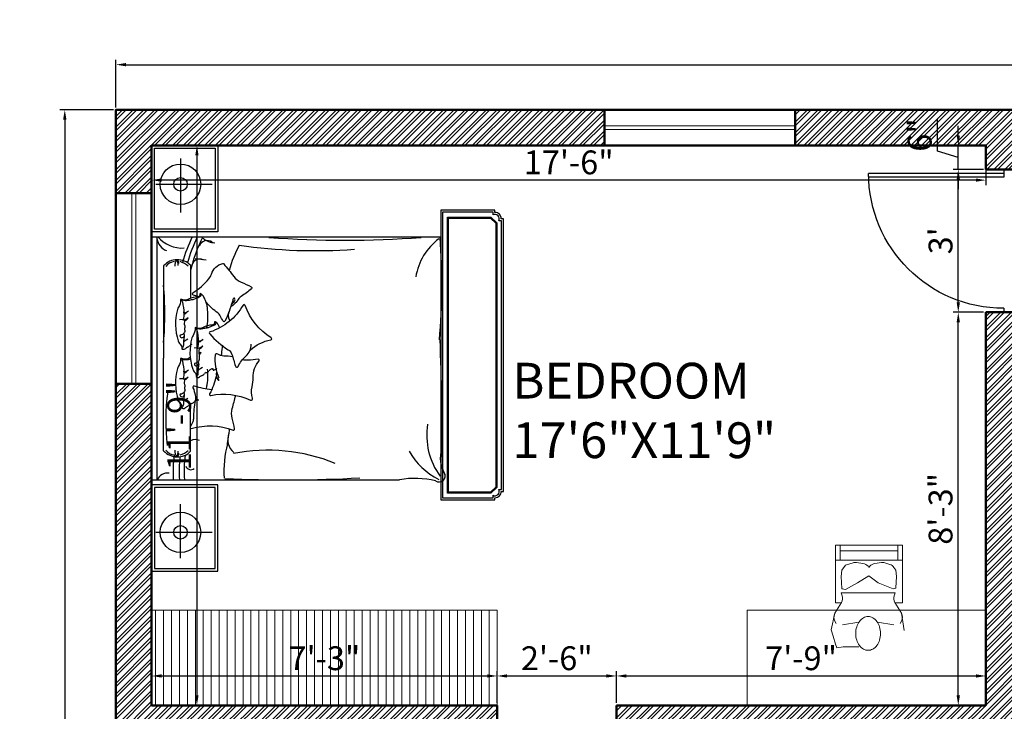
# Model space of a CAD drawing. Units: inches. Extents: x 3590 to 5167, y 65 to 1917.
# Tile 10 of 100: x 4396 to 4644, y 438 to 612. Entities that reach past the tile are written whole.
import ezdxf

# ---------------------------------------------------------------- set-up
doc = ezdxf.new("R2010")
doc.units = ezdxf.units.IN
for name, color, linetype, lineweight in [('A-ANNO-DIMS', 2, 'Continuous', 18), ('A-AREA-IDEN', 7, 'Continuous', 18), ('A-DOOR', 3, 'Continuous', 25), ('A-FURN', 21, 'Continuous', 18), ('A-GLAZ', 4, 'Continuous', 18), ('A-WALL', 7, 'Continuous', 50), ('A-WALL-PATT', 251, 'Continuous', 13)]:
    doc.layers.add(name, color=color, linetype=linetype, lineweight=lineweight)
for name, color, linetype in [('FUR', 42, 'Continuous'), ('HA-FUR', 8, 'Continuous'), ('HA-P', 8, 'Continuous'), ('SAN', 5, 'Continuous'), ('wood', 26, 'Continuous')]:
    doc.layers.add(name, color=color, linetype=linetype)
doc.styles.get("Standard").update_dxf_attribs({"font": 'arial.ttf'})
doc.dimstyles.new('ISO-25', dxfattribs={"dimtxt": 9, "dimasz": 2.5, "dimexe": 1.25, "dimexo": 0.625, "dimtad": 1, "dimdec": 1, "dimlunit": 3, "dimtxsty": 'Standard', "dimcen": 2.5, "dimadec": 0, "dimazin": 0, "dimtfac": 1, "dimtdec": 1, "dimtmove": 0, "dimatfit": 3, "dimfxl": 1, "dimarcsym": 0})

# ---------------------------------------------------------------- blocks, each defined once
blk = doc.blocks.new('*D279')
at = {"layer": 'A-ANNO-DIMS', "color": 0, "lineweight": -2, "transparency": 16777216}
for p, q in [((4420.27, 589.68), (4420.27, 601.68)), ((4422.77, 600.43), (5077.77, 600.43)), ((5080.27, 589.68), (5080.27, 601.68))]:
    blk.add_line(p, q, dxfattribs=at)
at = {"layer": 'A-ANNO-DIMS', "color": 0, "transparency": 16777216}
for points in [[(4422.77, 600.84), (4422.77, 600.01), (4420.27, 600.43)], [(5077.77, 600.84), (5077.77, 600.01), (5080.27, 600.43)]]:
    blk.add_solid(points, dxfattribs=at)
at = {"layer": 'Defpoints', "color": 0, "transparency": 16777216}
for p in [(5080.27, 600.43), (4420.27, 589.06), (5080.27, 589.06)]:
    blk.add_point(p, dxfattribs=at)
at = {"layer": 'A-ANNO-DIMS', "color": 0, "transparency": 16777216, "insert": (4750.27, 605.63), "char_height": 9, "attachment_point": 5}
blk.add_mtext("55'", dxfattribs=at)
blk = doc.blocks.new('*D280')
at = {"layer": 'A-ANNO-DIMS', "color": 0, "lineweight": -2, "transparency": 16777216}
for p, q in [((4419.65, 589.06), (4406.15, 589.06)), ((4407.4, 586.56), (4407.4, 111.56)), ((4419.65, 109.06), (4406.15, 109.06))]:
    blk.add_line(p, q, dxfattribs=at)
at = {"layer": 'A-ANNO-DIMS', "color": 0, "transparency": 16777216}
for points in [[(4406.98, 586.56), (4407.82, 586.56), (4407.4, 589.06)], [(4406.98, 111.56), (4407.82, 111.56), (4407.4, 109.06)]]:
    blk.add_solid(points, dxfattribs=at)
at = {"layer": 'Defpoints', "color": 0, "transparency": 16777216}
for p in [(4420.27, 589.06), (4407.4, 109.06), (4420.27, 109.06)]:
    blk.add_point(p, dxfattribs=at)
at = {"layer": 'A-ANNO-DIMS', "color": 0, "transparency": 16777216, "insert": (4402.18, 349.06), "char_height": 9, "attachment_point": 5, "rotation": 90}
blk.add_mtext("40'", dxfattribs=at)
blk = doc.blocks.new('D1')
for p, q in [((1, 0), (1, 34)), ((2, 0), (2, 33.99)), ((0, 0), (2, 0)), ((35, 0), (36, 0))]:
    blk.add_line(p, q)
at = {"ltscale": 0.5}
blk.add_arc((1, 0), 34, 0, 90, dxfattribs=at)
blk = doc.blocks.new('*D222')
at = {"layer": 'A-ANNO-DIMS', "color": 0, "lineweight": -2, "transparency": 16777216}
for p, q in [((4429.27, 579.43), (4429.27, 570.1)), ((4639.27, 579.43), (4639.27, 570.1)), ((4636.77, 571.35), (4431.77, 571.35))]:
    blk.add_line(p, q, dxfattribs=at)
at = {"layer": 'A-ANNO-DIMS', "color": 0, "transparency": 16777216}
for points in [[(4431.77, 571.77), (4431.77, 570.94), (4429.27, 571.35)], [(4636.77, 571.77), (4636.77, 570.94), (4639.27, 571.35)]]:
    blk.add_solid(points, dxfattribs=at)
at = {"layer": 'Defpoints', "color": 0, "transparency": 16777216}
for p in [(4429.27, 580.06), (4639.27, 580.06), (4429.27, 571.35)]:
    blk.add_point(p, dxfattribs=at)
at = {"layer": 'A-ANNO-DIMS', "color": 0, "transparency": 16777216, "insert": (4534.27, 575.04), "char_height": 6, "attachment_point": 5}
blk.add_mtext('17\'-6"', dxfattribs=at)
blk = doc.blocks.new('*D223')
at = {"layer": 'A-ANNO-DIMS', "color": 0, "lineweight": -2, "transparency": 16777216}
for p, q in [((4429.9, 580.06), (4441.91, 580.06)), ((4440.66, 577.56), (4440.66, 441.56)), ((4429.9, 439.06), (4441.91, 439.06))]:
    blk.add_line(p, q, dxfattribs=at)
at = {"layer": 'A-ANNO-DIMS', "color": 0, "transparency": 16777216}
for points in [[(4440.24, 577.56), (4441.08, 577.56), (4440.66, 580.06)], [(4440.24, 441.56), (4441.08, 441.56), (4440.66, 439.06)]]:
    blk.add_solid(points, dxfattribs=at)
at = {"layer": 'Defpoints', "color": 0, "transparency": 16777216}
for p in [(4429.27, 580.06), (4429.27, 439.06), (4440.66, 439.06)]:
    blk.add_point(p, dxfattribs=at)
at = {"layer": 'A-ANNO-DIMS', "color": 0, "transparency": 16777216, "insert": (4436.97, 509.56), "char_height": 6, "attachment_point": 5, "rotation": 90}
blk.add_mtext('11\'-9"', dxfattribs=at)
blk = doc.blocks.new('*D274')
at = {"layer": 'A-ANNO-DIMS', "color": 0, "lineweight": -2, "transparency": 16777216}
for p, q in [((4429.27, 439.68), (4429.27, 447.71)), ((4431.77, 446.46), (4513.77, 446.46)), ((4516.27, 439.68), (4516.27, 447.71))]:
    blk.add_line(p, q, dxfattribs=at)
at = {"layer": 'A-ANNO-DIMS', "color": 0, "transparency": 16777216}
for points in [[(4431.77, 446.88), (4431.77, 446.05), (4429.27, 446.46)], [(4513.77, 446.88), (4513.77, 446.05), (4516.27, 446.46)]]:
    blk.add_solid(points, dxfattribs=at)
at = {"layer": 'Defpoints', "color": 0, "transparency": 16777216}
for p in [(4516.27, 446.46), (4429.27, 439.06), (4516.27, 439.06)]:
    blk.add_point(p, dxfattribs=at)
at = {"layer": 'A-ANNO-DIMS', "color": 0, "transparency": 16777216, "insert": (4472.77, 450.15), "char_height": 6, "attachment_point": 5}
blk.add_mtext('7\'-3"', dxfattribs=at)
blk = doc.blocks.new('*D275')
at = {"layer": 'A-ANNO-DIMS', "color": 0, "lineweight": -2, "transparency": 16777216}
for p, q in [((4516.27, 439.68), (4516.27, 447.71)), ((4518.77, 446.46), (4543.77, 446.46)), ((4546.27, 439.68), (4546.27, 447.71))]:
    blk.add_line(p, q, dxfattribs=at)
at = {"layer": 'A-ANNO-DIMS', "color": 0, "transparency": 16777216}
for points in [[(4518.77, 446.88), (4518.77, 446.05), (4516.27, 446.46)], [(4543.77, 446.88), (4543.77, 446.05), (4546.27, 446.46)]]:
    blk.add_solid(points, dxfattribs=at)
at = {"layer": 'Defpoints', "color": 0, "transparency": 16777216}
for p in [(4546.27, 446.46), (4516.27, 439.06), (4546.27, 439.06)]:
    blk.add_point(p, dxfattribs=at)
at = {"layer": 'A-ANNO-DIMS', "color": 0, "transparency": 16777216, "insert": (4531.27, 450.15), "char_height": 6, "attachment_point": 5}
blk.add_mtext('2\'-6"', dxfattribs=at)
blk = doc.blocks.new('*D276')
at = {"layer": 'A-ANNO-DIMS', "color": 0, "lineweight": -2, "transparency": 16777216}
for p, q in [((4546.27, 439.68), (4546.27, 447.71)), ((4548.77, 446.46), (4636.77, 446.46)), ((4639.27, 439.68), (4639.27, 447.71))]:
    blk.add_line(p, q, dxfattribs=at)
at = {"layer": 'A-ANNO-DIMS', "color": 0, "transparency": 16777216}
for points in [[(4548.77, 446.88), (4548.77, 446.05), (4546.27, 446.46)], [(4636.77, 446.88), (4636.77, 446.05), (4639.27, 446.46)]]:
    blk.add_solid(points, dxfattribs=at)
at = {"layer": 'Defpoints', "color": 0, "transparency": 16777216}
for p in [(4639.27, 446.46), (4546.27, 439.06), (4639.27, 439.06)]:
    blk.add_point(p, dxfattribs=at)
at = {"layer": 'A-ANNO-DIMS', "color": 0, "transparency": 16777216, "insert": (4592.77, 450.15), "char_height": 6, "attachment_point": 5}
blk.add_mtext('7\'-9"', dxfattribs=at)
blk = doc.blocks.new('*D277')
at = {"layer": 'A-ANNO-DIMS', "color": 0, "lineweight": -2, "transparency": 16777216}
for p, q in [((4638.65, 538.06), (4631.09, 538.06)), ((4632.34, 441.56), (4632.34, 535.56)), ((4638.65, 439.06), (4631.09, 439.06))]:
    blk.add_line(p, q, dxfattribs=at)
at = {"layer": 'A-ANNO-DIMS', "color": 0, "transparency": 16777216}
for points in [[(4631.93, 535.56), (4632.76, 535.56), (4632.34, 538.06)], [(4631.93, 441.56), (4632.76, 441.56), (4632.34, 439.06)]]:
    blk.add_solid(points, dxfattribs=at)
at = {"layer": 'Defpoints', "color": 0, "transparency": 16777216}
for p in [(4632.34, 538.06), (4639.27, 538.06), (4639.27, 439.06)]:
    blk.add_point(p, dxfattribs=at)
at = {"layer": 'A-ANNO-DIMS', "color": 0, "transparency": 16777216, "insert": (4628.65, 488.56), "char_height": 6, "attachment_point": 5, "rotation": 90}
blk.add_mtext('8\'-3"', dxfattribs=at)
blk = doc.blocks.new('*D278')
at = {"layer": 'A-ANNO-DIMS', "color": 0, "lineweight": -2, "transparency": 16777216}
for p, q in [((4638.65, 574.06), (4631.09, 574.06)), ((4632.34, 540.56), (4632.34, 571.56)), ((4638.65, 538.06), (4631.09, 538.06))]:
    blk.add_line(p, q, dxfattribs=at)
at = {"layer": 'A-ANNO-DIMS', "color": 0, "transparency": 16777216}
for points in [[(4631.93, 571.56), (4632.76, 571.56), (4632.34, 574.06)], [(4631.93, 540.56), (4632.76, 540.56), (4632.34, 538.06)]]:
    blk.add_solid(points, dxfattribs=at)
at = {"layer": 'Defpoints', "color": 0, "transparency": 16777216}
for p in [(4632.34, 574.06), (4639.27, 574.06), (4639.27, 538.06)]:
    blk.add_point(p, dxfattribs=at)
at = {"layer": 'A-ANNO-DIMS', "color": 0, "transparency": 16777216, "insert": (4628.65, 556.06), "char_height": 6, "attachment_point": 5, "rotation": 90}
blk.add_mtext("3'", dxfattribs=at)
blk = doc.blocks.new('*D269')
at = {"layer": 'A-ANNO-DIMS', "color": 0, "lineweight": -2, "transparency": 16777216}
for p, q in [((4627.09, 578.64), (4627.09, 586.81)), ((4632.34, 582.56), (4632.34, 585.06)), ((4638.65, 580.06), (4631.09, 580.06)), ((4632.34, 574.06), (4632.34, 580.06)), ((4632.34, 574.06), (4632.34, 580.06)), ((4632.34, 577.06), (4627.09, 578.64)), ((4638.65, 574.06), (4631.09, 574.06)), ((4632.34, 571.56), (4632.34, 569.06))]:
    blk.add_line(p, q, dxfattribs=at)
at = {"layer": 'A-ANNO-DIMS', "color": 0, "transparency": 16777216}
for points in [[(4631.93, 582.56), (4632.76, 582.56), (4632.34, 580.06)], [(4631.93, 571.56), (4632.76, 571.56), (4632.34, 574.06)]]:
    blk.add_solid(points, dxfattribs=at)
at = {"layer": 'Defpoints', "color": 0, "transparency": 16777216}
for p in [(4632.34, 580.06), (4639.27, 580.06), (4639.27, 574.06)]:
    blk.add_point(p, dxfattribs=at)
at = {"layer": 'A-ANNO-DIMS', "color": 0, "transparency": 16777216, "insert": (4623.4, 582.72), "char_height": 6, "attachment_point": 5, "rotation": 90}
blk.add_mtext('6"', dxfattribs=at)
blk = doc.blocks.new('A$C0A42580C')
at = {"layer": 'SAN'}
for p, q in [((0.2873, 0.0301), (0.2873, 0.4484)), ((2.8678, 0.0301), (2.8678, 0.4484)), ((0.0949, 0.2135), (0.4958, 0.2135)), ((3.0601, 0.2135), (2.6592, 0.2135))]:
    blk.add_line(p, q, dxfattribs=at)
for centre, radius in [((0.2873, 0.2135), 0.15), ((2.8678, 0.2135), 0.15), ((0.2873, 0.2135), 0.05), ((2.8678, 0.2135), 0.05)]:
    blk.add_circle(centre, radius, dxfattribs=at)
at = {"layer": 'wood'}
for p, q in [((0.6775, 0.8851), (0.6775, 2.1392)), ((2.4775, 0.8016), (2.4775, 1.838)), ((2.4775, 0), (2.4775, 0.8016)), ((1.6633, 0.3438), (1.6434, 0.3761)), ((1.5, 0.3423), (1.5016, 0.3142)), ((0.888, 0.289), (1.1327, 0.289)), ((1.2906, 0.2348), (1.2921, 0.2067)), ((1.4538, 0.2362), (1.434, 0.2685)), ((1.7287, 0.2348), (1.7302, 0.2067)), ((1.8919, 0.2362), (1.8721, 0.2685)), ((2.267, 0.289), (1.9163, 0.289)), ((0.8909, 0.089), (1.5775, 0.089)), ((2.2642, 0.089), (1.5775, 0.089)), ((0.6775, 0.039), (2.4775, 0.039)), ((0.6775, 0), (2.4775, 0))]:
    blk.add_line(p, q, dxfattribs=at)
blk.add_lwpolyline([(0.6775, 0), (0.6775, 0.8851)], dxfattribs=at)
for points in [[(1.516, 0.7294, -0.128392), (1.4401, 0.8834, 0.70791), (1.427, 0.8863, -0.16964), (1.1848, 0.6919, 0.664036), (1.184, 0.6776, -0.184649), (1.3819, 0.4332, 0.662242), (1.3969, 0.4309, 0.078539), (1.5137, 0.5669, -0.1736), (1.5484, 0.5947, -0.02159), (1.6357, 0.6205, 0.697276), (1.6379, 0.6405, -0.093019), (1.5606, 0.699, 0.216632), (1.4719, 0.7371, -2.511293)], [(1.1211, 0.3454, 0.032543), (1.1095, 0.3091, -0.658965), (1.0917, 0.3063, 0.074753), (0.9887, 0.4234, 0.100988), (0.953, 0.4429, -0.270711), (0.8753, 0.5273, -0.276825), (0.8775, 0.5337, -0.014937), (0.9701, 0.6081, 0.134834), (1.0135, 0.6643, -0.023706), (1.0474, 0.7372, -0.664036), (1.0616, 0.7394, -0.035987), (1.119, 0.6627, 0.118631), (1.1415, 0.6412, -0.132738), (1.1955, 0.5864)], [(1.6795, 0.4818, 0.263265), (1.7191, 0.4839, -0.026108), (1.743, 0.4973, 0.027613), (1.7137, 0.4764, -0.089259), (1.8403, 0.429, 0.662242), (1.8528, 0.4376, -0.162037), (1.8882, 0.732, 0.676499), (1.8733, 0.748, -0.160513), (1.7901, 0.7439, 0.07473), (1.7202, 0.7523, -0.187721), (1.5966, 0.7963, 0.70791), (1.5851, 0.7895, -0.010003), (1.5921, 0.7143, -0.07079), (1.5891, 0.6719, 0.099539)], [(1.1759, 0.5928, 0.013884), (1.1549, 0.6131, 0.174178), (1.1437, 0.6177, 0.104076), (1.1358, 0.6165, 0.389829), (1.1324, 0.6097, 0.296089), (1.1415, 0.6019, -0.036701), (1.1572, 0.5985, -0.040547), (1.3022, 0.543, -0.70791), (1.3021, 0.5296, -0.016811), (1.2631, 0.5085, 0.11866), (1.2414, 0.4904, -0.048791), (1.1649, 0.4055, 0.103757)], [(1.5674, 0.601, 0.057807), (1.5606, 0.5339, -0.173425), (1.5457, 0.49, 0.589988), (1.5538, 0.4706, 0.137312), (1.7236, 0.4985, 0.137312)], [(1.8113, 0.4446, -0.069098), (1.7831, 0.3187, 0.658965), (1.7961, 0.3062, -0.049789), (1.8516, 0.3234, -0.103757), (1.8905, 0.3233, 0.055725), (2.0203, 0.3103, -0.11866), (2.0478, 0.304, 0.016811), (2.0881, 0.2856, 0.70791), (2.0989, 0.2936, -0.16964), (2.1104, 0.604, 0.664036), (2.1001, 0.6139, 0.023706), (2.0214, 0.597, -0.134834), (1.9505, 0.5976, 0.012748), (1.8522, 0.6228)], [(1.3107, 0.4764, 0.145733), (1.3069, 0.4677, 0.488583), (1.3089, 0.4657, -0.012138), (1.3131, 0.4661, -0.125673), (1.3213, 0.4646, -0.750706)], [(1.3153, 0.4751, -0.274893), (1.3379, 0.4529, 0.051436), (1.3468, 0.4293, -0.086628), (1.3532, 0.4078, 0.040196), (1.3593, 0.3772, -0.184744), (1.3556, 0.3344, -2.554464)], [(1.317, 0.4683, -0.060098), (1.3283, 0.4571, -0.16247), (1.3313, 0.4487, 0.120018), (1.3493, 0.3815, -0.060072), (1.3541, 0.3695, -0.13107), (1.3541, 0.3395, -0.024415), (1.3534, 0.3373, 0.070398), (1.3503, 0.3233, 0.528689), (1.3524, 0.3216, -0.069388), (1.3557, 0.3222, -0.158233), (1.4075, 0.3065, 0.085461), (1.4255, 0.2981, 0.147196), (1.6571, 0.3041, 0.10985), (1.6823, 0.3191, -0.179095), (1.7126, 0.3319, -2.318897)], [(1.1013, 0.3688, 0.145733), (1.0975, 0.3601, 0.488583), (1.0995, 0.3581, -0.012138), (1.1036, 0.3585, -0.125673), (1.1119, 0.357, -0.750706)], [(1.1059, 0.3675, -0.274893), (1.1285, 0.3453, 0.051436), (1.1373, 0.3217, -0.086628), (1.1438, 0.3003, 0.040196), (1.1499, 0.2696, -0.184744), (1.1462, 0.2269, -2.554464)], [(1.4359, 0.3803, -0.198519), (1.452, 0.3494, 0.826402), (1.4558, 0.349, 0.095956), (1.4561, 0.3528, 0.242899), (1.4461, 0.3686, -17.523452)], [(1.5447, 0.3525, -0.083557), (1.507, 0.3546, 0.203162), (1.4851, 0.3792, -0.208037), (1.5043, 0.3409, 0.124669), (1.4432, 0.3469, 0.965934)], [(1.5394, 0.3688, 0.145733), (1.5356, 0.3601, 0.488583), (1.5376, 0.3581, -0.012138), (1.5418, 0.3585, -0.125673), (1.55, 0.357, -0.750706)], [(1.1076, 0.3607, -0.060098), (1.1189, 0.3495, -0.16247), (1.1219, 0.3411, 0.120018), (1.1399, 0.2739, -0.060072), (1.1447, 0.2619, -0.13107), (1.1447, 0.2319, -0.024415), (1.144, 0.2297, 0.070398), (1.1409, 0.2157, 0.528689), (1.143, 0.2141, -0.069388), (1.1463, 0.2146, -0.158233), (1.1981, 0.1989, 0.085461), (1.2161, 0.1905, 0.147196), (1.4477, 0.1965, 0.10985), (1.4728, 0.2115, -0.179095), (1.5032, 0.2244, -2.318897)], [(1.3509, 0.3219, -0.117141), (1.3688, 0.335, -0.025084), (1.4533, 0.348, 0.033691)], [(1.5447, 0.3525, -0.008229), (1.5728, 0.3519, 0.033691)], [(1.5728, 0.3519, -0.46905), (1.6152, 0.321, 0.420988), (1.62, 0.3169, 0.857652), (1.6221, 0.3484, 0.548526)], [(1.603, 0.3451, -0.099719), (1.6221, 0.3484, 0.102691)], [(1.6214, 0.3487, -0.010168), (1.6558, 0.3447, 0.033691), (1.6907, 0.3423, -0.220869), (1.7148, 0.3311, -0.288972)], [(1.1415, 0.2143, -0.117141), (1.1594, 0.2274, -0.025084), (1.2439, 0.2405, 0.033691)], [(1.2265, 0.2728, -0.198519), (1.2426, 0.2418, 0.826402), (1.2463, 0.2415, 0.095956), (1.2467, 0.2452, 0.242899), (1.2366, 0.2611, -17.523452)], [(1.3353, 0.2449, -0.083557), (1.2976, 0.247, 0.203162), (1.2757, 0.2717, -0.208037), (1.2948, 0.2333, 0.124669), (1.2338, 0.2393, 0.965934)], [(1.3353, 0.2449, -0.008229), (1.3633, 0.2443, 0.033691)], [(1.3633, 0.2443, -0.46905), (1.4058, 0.2134, 0.420988), (1.4106, 0.2093, 0.857652), (1.4127, 0.2408, 0.548526)], [(1.3936, 0.2375, -0.099719), (1.4127, 0.2408, 0.102691)], [(1.412, 0.2411, -0.010168), (1.4464, 0.2371, 0.033691), (1.4812, 0.2348, -0.220869), (1.5054, 0.2235, -0.288972)], [(1.5721, 0.286, 0.022869), (1.578, 0.2739, -0.060072), (1.5828, 0.2619, -0.13107), (1.5828, 0.2319, -0.024415), (1.5821, 0.2297, 0.070398), (1.579, 0.2157, 0.528689), (1.5811, 0.2141, -0.069388), (1.5844, 0.2146, -0.158233), (1.6362, 0.1989, 0.085461), (1.6542, 0.1905, 0.147196), (1.8858, 0.1965, 0.10985), (1.911, 0.2115, -0.179095), (1.9413, 0.2244, -2.318897)], [(1.5796, 0.2143, -0.117141), (1.5975, 0.2274, -0.025084), (1.682, 0.2405, 0.033691)], [(1.5838, 0.2873, 0.023398), (1.588, 0.2696, -0.184744), (1.5843, 0.2269, -2.554464)], [(1.6646, 0.2728, -0.198519), (1.6807, 0.2418, 0.826402), (1.6845, 0.2415, 0.095956), (1.6848, 0.2452, 0.242899), (1.6748, 0.2611, -17.523452)], [(1.7734, 0.2449, -0.083557), (1.7357, 0.247, 0.203162), (1.7138, 0.2717, -0.208037), (1.733, 0.2333, 0.124669), (1.6719, 0.2393, 0.965934)], [(1.7734, 0.2449, -0.008229), (1.8015, 0.2443, 0.033691)], [(1.8015, 0.2443, -0.46905), (1.8439, 0.2134, 0.420988), (1.8487, 0.2093, 0.857652), (1.8508, 0.2408, 0.548526)], [(1.8317, 0.2375, -0.099719), (1.8508, 0.2408, 0.102691)], [(1.8501, 0.2411, -0.010168), (1.8845, 0.2371, 0.033691), (1.9193, 0.2348, -0.220869), (1.9435, 0.2235, -0.288972)]]:
    blk.add_lwpolyline(points, format="xyb", dxfattribs=at)
for points in [[(0.64, 0), (0, 0), (0, 0.49), (0.64, 0.49)], [(0.62, 0.02), (0.02, 0.02), (0.02, 0.47), (0.62, 0.47)], [(2.515, 0), (3.155, 0), (3.155, 0.49), (2.515, 0.49)], [(2.535, 0.02), (3.135, 0.02), (3.135, 0.47), (2.535, 0.47)]]:
    blk.add_lwpolyline(points, close=True, dxfattribs=at)
for centre, radius, start, end in [((1.0344, -2.14), 4.292, 84.56078, 94.7164), ((1.0494, 2.4026), 0.4515, 217.47941, 260.35986), ((2.0208, -11.0786), 13.2288, 88.75549, 92.51133), ((2.1491, 2.5471), 0.5083, 260.65485, 306.44155), ((2.3125, 2.3833), 0.2443, 254.1515, 300.95574), ((2.0168, 2.3573), 0.5127, 299.08175, 333.44367), ((2.4501, 2.1309), 0.0445, 324.18954, 118.92203), ((3.1371, 1.9502), 0.669, 166.6404, 189.65708), ((-7.0839, 1.4328), 7.7858, 355.84817, 4.15183), ((-7.2439, 0.9937), 9.7233, 357.34474, 3.23068), ((-3.167, 1.2143), 3.9465, 351.77286, 4.18386), ((3.5803, 0.8622), 1.3213, 157.81295, 191.15154), ((1.1611, 1.4181), 0.8768, 241.21362, 254.41879), ((2.181, 0.6859), 0.1221, 247.37754, 321.13165), ((1.2583, 0.6364), 0.0695, 238.58923, 301.92671), ((1.4714, 0.0722), 0.4528, 80.62397, 88.74059), ((1.4035, -0.3388), 0.8693, 79.71489, 80.62397), ((1.7861, -2.1601), 2.7557, 80.89877, 83.46656), ((2.4192, 1.3819), 0.8461, 255.77539, 273.25587), ((0.5904, 0.4689), 0.13, 317.38218, 359.70393), ((0.7723, 0.4131), 0.0674, 147.68233, 245.79865), ((1.3546, 0.4469), 0.0529, 114.21284, 146.15395), ((2.6126, -2.3504), 3.1201, 113.83178, 114.21284), ((1.6301, 0.4539), 0.0342, 31.14095, 54.95422), ((1.6709, 0.4489), 0.0156, 131.9623, 212.08127), ((1.6729, 0.4422), 0.0178, 140.41793, 157.63267), ((1.7235, 0.4818), 0.0777, 212.08127, 227.364), ((1.6635, 0.4499), 0.00568, 95.52245, 140.41793), ((1.5664, 0.4154), 0.1086, 24.20989, 31.14095), ((1.6627, 0.4587), 0.00309, 275.52245, 24.20989), ((1.1611, 1.3191), 1.0568, 242.76671, 257.10398), ((0.0312, 0.4583), 0.8174, 350.42368, 356.2506), ((0.9021, 0.3562), 0.0605, 155.8342, 254.41058), ((1.1452, 0.3394), 0.0529, 114.21284, 146.15395), ((2.4032, -2.458), 3.1201, 113.55686, 114.21284), ((1.2046, 0.2912), 0.121, 99.42032, 113.55686), ((1.2774, -0.1478), 0.5659, 95.90379, 99.42032), ((1.2626, -0.005), 0.4223, 88.74059, 95.90379), ((1.2619, -0.0354), 0.4528, 80.62397, 88.74059), ((1.1941, -0.4464), 0.8693, 79.45871, 80.62397), ((1.4207, 0.3463), 0.0342, 31.14095, 54.95422), ((1.7007, -0.005), 0.4223, 88.74059, 95.90379), ((1.6391, 0.3902), 0.0469, 17.32618, 47.364), ((1.7106, 0.4125), 0.028, 197.32618, 226.17302), ((1.6431, 0.3422), 0.0695, 26.61764, 46.17302), ((1.8202, 0.431), 0.1287, 206.61764, 215.96192), ((1.7001, -0.0354), 0.4528, 80.62397, 88.74059), ((1.6322, -0.4464), 0.8693, 78.43923, 80.62397), ((1.1611, 1.3191), 1.0937, 243.75553, 254.4906), ((1.1611, 1.2816), 1.0937, 243.75553, 254.38927), ((1.4614, 0.3413), 0.0156, 131.9623, 212.08127), ((1.4635, 0.3347), 0.0178, 140.41793, 157.63267), ((1.4541, 0.3424), 0.00568, 95.52245, 140.41793), ((1.357, 0.3078), 0.1086, 24.20989, 31.14095), ((1.4533, 0.3511), 0.00309, 275.52245, 24.20989), ((1.5012, 0.305), 0.028, 197.32618, 226.17302), ((1.715, 0.3349), 0.00379, 207.1817, 328.02977), ((1.6975, 0.3419), 0.023, 350.76434, 35.96192), ((1.7058, 0.3406), 0.0145, 328.02977, 350.76434), ((1.9016, 0.3347), 0.0178, 140.41793, 157.63267), ((1.9522, 0.3743), 0.0777, 212.08127, 227.364), ((1.8922, 0.3424), 0.00568, 95.52245, 140.41793), ((1.8678, 0.2827), 0.0469, 17.32618, 47.364), ((1.9393, 0.305), 0.028, 197.32618, 226.17302), ((2.2511, 0.3256), 0.071, 155.86842, 211.04513), ((2.3616, 0.2915), 0.0419, 290.78583, 35.36309), ((0.5293, 0.2241), 0.2307, 309.63048, 4.27465), ((0.9846, 0.1903), 0.1381, 134.39284, 227.23745), ((0.9986, 0.1735), 0.1427, 136.58239, 164.9725), ((1.4337, 0.2347), 0.0695, 26.61764, 46.17302), ((1.6108, 0.3235), 0.1287, 206.61764, 215.96192), ((1.5055, 0.2273), 0.00379, 207.1817, 328.02977), ((1.4881, 0.2344), 0.023, 350.76434, 35.96192), ((1.4964, 0.233), 0.0145, 328.02977, 350.76434), ((1.8718, 0.2347), 0.0695, 26.61764, 46.17302), ((2.0489, 0.3235), 0.1287, 206.61764, 215.96192), ((1.9436, 0.2273), 0.00379, 207.1817, 328.02977), ((1.9262, 0.2344), 0.023, 350.76434, 35.96192), ((1.9345, 0.233), 0.0145, 328.02977, 350.76434), ((2.1565, 0.1735), 0.1427, 15.0275, 43.41761), ((2.1704, 0.1903), 0.1381, 312.76255, 45.60716), ((2.4192, 1.2667), 1.0261, 263.09035, 273.25587), ((0.8396, 0.185), 0.0112, 314.89662, 45.10338), ((0.8413, 0.1846), 0.0128, 299.47062, 57.44416), ((0.8844, 0.2286), 0.0569, 229.70587, 281.11527), ((0.8802, 0.1371), 0.0592, 81.47786, 123.11925), ((0.8698, 0.1793), 0.0229, 77.14902, 159.1786), ((0.9466, 0.1765), 0.0862, 185.53723, 234.68694), ((2.2085, 0.1765), 0.0862, 305.31306, 354.46277), ((2.2706, 0.2286), 0.0569, 258.88473, 310.29413), ((2.2749, 0.1371), 0.0592, 56.88075, 98.52214), ((2.2853, 0.1793), 0.0229, 20.8214, 102.85098), ((2.4192, 1.2218), 1.0629, 263.23622, 273.25587), ((2.3138, 0.1846), 0.0128, 122.55584, 240.52938), ((2.3154, 0.185), 0.0112, 134.89662, 225.10338), ((2.4192, 1.2667), 1.0629, 263.94374, 273.25587), ((0.6729, 0.151), 0.1135, 279.23824, 338.73819), ((1.2481, -2.5919), 2.6893, 85.4722, 94.5278), ((2.0447, 1.7022), 1.5979, 262.13639, 276.48786), ((2.508, 0.1152), 0.0792, 169.94668, 248.24015)]:
    blk.add_arc(centre, radius, start, end, dxfattribs=at)
blk = doc.blocks.new('A$C623F1DA0')
at = {"layer": 'FUR'}
blk.add_lwpolyline([(0.628, 2.912, 0.414214), (0.562, 2.978), (0.562, 3), (0, 3), (0, 0), (0.562, 0), (0.562, 0.022, 0.414214), (0.628, 0.088), (0.65, 0.088), (0.65, 2.912)], format="xyb", close=True, dxfattribs=at)
at = {"layer": 'HA-FUR'}
blk.add_lwpolyline([(0.603, 2.892, 0.710288), (0.542, 2.953), (0.542, 2.98), (0.02, 2.98), (0.02, 0.02), (0.542, 0.02), (0.542, 0.047, 0.710288), (0.603, 0.108), (0.63, 0.108), (0.63, 2.892)], format="xyb", close=True, dxfattribs=at)
at = {"layer": 'HA-P'}
for points in [[(0.07, 2.93), (0.521, 2.93), (0.58, 2.871), (0.58, 0.129), (0.521, 0.07), (0.07, 0.07)], [(0.08, 2.92), (0.517, 2.92), (0.57, 2.867), (0.57, 0.133), (0.517, 0.08), (0.08, 0.08)]]:
    blk.add_lwpolyline(points, close=True, dxfattribs=at)

msp = doc.modelspace()

# ---------------------------------------------------------------- hatches: boundary and pattern name
at = {"layer": 'A-WALL-PATT', "transparency": 33554687}
h = msp.add_hatch(dxfattribs=at)
h.set_pattern_fill('ANSI32', color=256, scale=0.2)
h.set_pattern_definition([(45, (0, -1216.9392), (-1.3470384, 1.3470384), []), (45, (0.898, -1216.9392), (-1.3470384, 1.3470384), [])])
h.paths.add_polyline_path([(4684.27, 589.06), (4591.27, 589.06), (4591.27, 580.06), (4639.27, 580.06), (4639.27, 574.06), (4648.27, 574.06), (4648.27, 580.06), (4684.27, 580.06)])
h.paths.add_polyline_path([(4543.27, 589.06), (4420.27, 589.06), (4420.27, 568.06), (4429.27, 568.06), (4429.27, 580.06), (4445.92, 580.06), (4543.27, 580.06)])
h.paths.add_polyline_path([(4828.27, 589.06), (4744.27, 589.06), (4744.27, 580.06), (4828.27, 580.06)])
h.paths.add_polyline_path([(4648.27, 538.06), (4639.27, 538.06), (4639.27, 439.06), (4546.27, 439.06), (4546.27, 433.06), (4549.27, 433.06), (4549.27, 337.06), (4429.27, 337.06), (4429.27, 367.06), (4420.27, 367.06), (4420.27, 322.06), (4429.27, 322.06), (4429.27, 328.06), (4639.27, 328.06), (4639.27, 322.06), (4648.27, 322.06), (4648.27, 343.06), (4639.27, 343.06), (4639.27, 337.06), (4555.27, 337.06), (4555.27, 433.06), (4639.27, 433.06), (4639.27, 373.06), (4648.27, 373.06)])
h.paths.add_polyline_path([(4516.27, 439.06), (4429.27, 439.06), (4429.27, 520.06), (4420.27, 520.06), (4420.27, 403.06), (4429.27, 403.06), (4429.27, 433.06), (4516.27, 433.06)], flags=17)
h.paths.add_polyline_path([(5080.27, 589.06), (4888.27, 589.06), (4888.27, 580.06), (4924.27, 580.06), (4924.27, 538.06), (4933.27, 538.06), (4933.27, 580.06), (5071.27, 580.06), (5071.27, 118.06), (4933.27, 118.06), (4933.27, 349.06), (4924.27, 349.06), (4924.27, 118.06), (4898.77, 118.06), (4898.77, 109.06), (5080.27, 109.06)])
h.paths.add_polyline_path([(4933.27, 502.06), (4924.27, 502.06), (4924.27, 421.06), (4933.27, 421.06)], flags=17)
h.paths.add_polyline_path([(4802.77, 118.06), (4777.27, 118.06), (4777.27, 286.06), (4756.27, 286.06), (4756.27, 277.06), (4768.27, 277.06), (4768.27, 214.06), (4696.27, 214.06), (4696.27, 277.06), (4708.27, 277.06), (4708.27, 286.06), (4639.27, 286.06), (4639.27, 277.06), (4687.27, 277.06), (4687.27, 214.06), (4681.27, 214.06), (4681.27, 205.06), (4768.27, 205.06), (4768.27, 118.06), (4726.27, 118.06), (4726.27, 109.06), (4802.77, 109.06)])
h.paths.add_polyline_path([(4690.27, 118.06), (4648.27, 118.06), (4648.27, 135.93), (4648.27, 205.06), (4651.27, 205.06), (4651.27, 214.06), (4639.27, 214.06), (4639.27, 118.06), (4633.27, 118.06), (4633.27, 109.06), (4690.27, 109.06)])
h.paths.add_polyline_path([(4585.27, 118.06), (4584.72, 118.06), (4429.27, 118.06), (4429.27, 274.06), (4420.27, 274.06), (4420.27, 109.06), (4585.27, 109.06)])

# ---------------------------------------------------------------- linework, layer by layer
at = {"layer": 'A-FURN'}
for p, q in [((4601.42, 479.38), (4601.42, 464.87)), ((4618.26, 479.38), (4601.42, 479.38)), ((4602.57, 475.61), (4602.57, 479.38)), ((4617.16, 475.61), (4617.16, 479.38)), ((4618.26, 464.87), (4618.26, 479.38)), ((4617.16, 477.94), (4602.57, 477.94)), ((4618.26, 475.61), (4601.42, 475.61)), ((4603.03, 473.11), (4603.92, 474.36)), ((4603.92, 474.36), (4605.85, 474.95)), ((4606.68, 475.02), (4608.32, 474.82)), ((4609.62, 474.09), (4609.84, 473.82)), ((4610.05, 474.09), (4609.84, 473.82)), ((4613, 475.02), (4611.35, 474.82)), ((4615.11, 474.56), (4613.83, 474.95)), ((4616.65, 473.11), (4616.14, 473.82)), ((4602.85, 471.5), (4603.03, 473.11)), ((4603.03, 468.51), (4602.85, 471.5)), ((4609.84, 471.68), (4606.97, 469.88)), ((4612.17, 469.88), (4609.84, 471.68)), ((4616.82, 471.5), (4616.65, 473.11)), ((4616.66, 468.66), (4616.82, 471.5)), ((4606.97, 469.88), (4603.92, 468.27)), ((4615.93, 468.45), (4612.17, 469.88)), ((4616.6, 468.58), (4615.93, 468.45)), ((4602.85, 467.38), (4616.47, 467.38)), ((4616.47, 467.38), (4602.85, 467.38)), ((4602.85, 467.38), (4603.1, 466.63)), ((4603.92, 468.27), (4603.09, 468.44)), ((4616.47, 467.38), (4616.22, 466.63)), ((4602.92, 464.98), (4601.29, 462.27)), ((4601.42, 464.87), (4602.85, 464.87)), ((4616.4, 464.98), (4618.03, 462.27)), ((4616.47, 464.87), (4618.26, 464.87)), ((4429.27, 463.06), (4516.27, 463.06)), ((4430.27, 463.06), (4430.27, 439.06)), ((4432.27, 463.06), (4432.27, 439.06)), ((4434.27, 463.06), (4434.27, 439.06)), ((4436.27, 463.06), (4436.27, 439.06)), ((4438.27, 463.06), (4438.27, 439.06)), ((4440.27, 463.06), (4440.27, 439.06)), ((4442.27, 463.06), (4442.27, 439.06)), ((4444.27, 463.06), (4444.27, 439.06)), ((4446.27, 463.06), (4446.27, 439.06)), ((4448.27, 463.06), (4448.27, 439.06)), ((4450.27, 463.06), (4450.27, 439.06)), ((4452.27, 463.06), (4452.27, 439.06)), ((4454.27, 463.06), (4454.27, 439.06)), ((4456.27, 463.06), (4456.27, 439.06)), ((4458.27, 463.06), (4458.27, 439.06)), ((4460.27, 463.06), (4460.27, 439.06)), ((4462.27, 463.06), (4462.27, 439.06)), ((4464.27, 463.06), (4464.27, 439.06)), ((4466.27, 463.06), (4466.27, 439.06)), ((4468.27, 463.06), (4468.27, 439.06)), ((4470.27, 463.06), (4470.27, 439.06)), ((4472.27, 463.06), (4472.27, 439.06)), ((4474.27, 463.06), (4474.27, 439.06)), ((4476.27, 463.06), (4476.27, 439.06)), ((4478.27, 463.06), (4478.27, 439.06)), ((4480.27, 463.06), (4480.27, 439.06)), ((4482.27, 463.06), (4482.27, 439.06)), ((4484.27, 463.06), (4484.27, 439.06)), ((4486.27, 463.06), (4486.27, 439.06)), ((4488.27, 463.06), (4488.27, 439.06)), ((4490.27, 463.06), (4490.27, 439.06)), ((4492.27, 463.06), (4492.27, 439.06)), ((4494.27, 463.06), (4494.27, 439.06)), ((4496.27, 463.06), (4496.27, 439.06)), ((4498.27, 463.06), (4498.27, 439.06)), ((4500.27, 463.06), (4500.27, 439.06)), ((4502.27, 463.06), (4502.27, 439.06)), ((4504.27, 463.06), (4504.27, 439.06)), ((4506.27, 463.06), (4506.27, 439.06)), ((4508.27, 463.06), (4508.27, 439.06)), ((4510.27, 463.06), (4510.27, 439.06)), ((4512.27, 463.06), (4512.27, 439.06)), ((4514.27, 463.06), (4514.27, 439.06)), ((4516.27, 463.06), (4516.27, 439.06)), ((4579.23, 463.06), (4639.27, 463.06)), ((4579.23, 463.06), (4579.23, 439.06)), ((4618.03, 462.27), (4618.68, 457.92)), ((4601.26, 460.29), (4601.6, 459.68)), ((4603.21, 459.32), (4607.33, 460.04)), ((4616.11, 459.32), (4611.99, 460.04)), ((4618.06, 460.29), (4617.72, 459.68))]:
    msp.add_line(p, q, dxfattribs=at)
msp.add_lwpolyline([(4601.29, 462.27), (4600.34, 458.07), (4600.88, 456.45), (4601.42, 454.48), (4601.77, 453.59), (4603.39, 453.77), (4605, 453.77), (4607.33, 453.77)], dxfattribs=at)
msp.add_lwpolyline([(4612.77, 457.17, 0.07405), (4612.52, 458.85, 0.084801), (4611.86, 460.17, 0.106336), (4610.79, 461.12, 0.128955), (4609.65, 461.42, 0.128955), (4608.5, 461.12, 0.106336), (4607.44, 460.17, 0.084801), (4606.77, 458.85, 0.07405), (4606.52, 457.17, 0.07405), (4606.77, 455.49, 0.084801), (4607.44, 454.17, 0.106336), (4608.5, 453.22, 0.128955), (4609.65, 452.92, 0.128955), (4610.79, 453.22, 0.106336), (4611.86, 454.17, 0.084801), (4612.52, 455.49, 0.07405)], format="xyb", close=True, dxfattribs=at)
for centre, radius, start, end in [((4606.43, 473.06), 1.98, 82.8785, 107.0946), ((4608.07, 472.85), 1.98, 38.6739, 82.8785), ((4611.6, 472.85), 1.98, 97.1215, 141.3261), ((4613.24, 473.06), 1.98, 72.9054, 97.1215), ((4614.53, 472.66), 1.98, 35.5514, 72.9054), ((4603.1, 468.52), 0.0779, 183.3682, 258.6956), ((4603.1, 468.52), 0.0779, 183.3682, 258.6956), ((4616.58, 468.66), 0.0779, 281.3044, 356.6318), ((4601.22, 466), 1.98, 329.0235, 18.4436), ((4618.1, 466), 1.98, 161.5564, 210.9765), ((4602.99, 461.25), 1.98, 149.0235, 209.0669), ((4616.32, 461.25), 1.98, 330.9331, 30.9765)]:
    msp.add_arc(centre, radius, start, end, dxfattribs=at)
at = {"layer": 'A-GLAZ'}
for p, q in [((4591.27, 585.06), (4543.27, 585.06)), ((4591.27, 584.06), (4543.27, 584.06)), ((4424.27, 520.06), (4424.27, 568.06)), ((4425.27, 520.06), (4425.27, 568.06))]:
    msp.add_line(p, q, dxfattribs=at)
at = {"layer": 'A-WALL'}
for p, q in [((4543.27, 580.06), (4543.27, 589.06)), ((4591.27, 580.06), (4591.27, 589.06)), ((4429.27, 580.06), (4639.27, 580.06)), ((4429.27, 439.06), (4429.27, 580.06)), ((4639.27, 574.06), (4639.27, 580.06)), ((4639.27, 574.06), (4648.27, 574.06)), ((4429.27, 568.06), (4420.27, 568.06)), ((4639.27, 538.06), (4648.27, 538.06)), ((4639.27, 439.06), (4639.27, 538.06)), ((4429.27, 520.06), (4420.27, 520.06)), ((4429.27, 439.06), (4516.27, 439.06)), ((4516.27, 433.06), (4516.27, 439.06)), ((4546.27, 439.06), (4639.27, 439.06)), ((4546.27, 433.06), (4546.27, 439.06))]:
    msp.add_line(p, q, dxfattribs=at)
msp.add_lwpolyline([(5080.27, 589.06), (5080.27, 109.06), (4420.27, 109.06), (4420.27, 589.06)], close=True, dxfattribs=at)

# ---------------------------------------------------------------- block references
at = {"layer": 'A-DOOR', "xscale": -1, "rotation": 90}
msp.add_blockref('D1', (4643.77, 574.06), dxfattribs=at)
at = {"layer": 'A-FURN', "xscale": 33.96864568351422, "yscale": 33.96864568351422, "zscale": 33.96864568351422, "rotation": 270}
msp.add_blockref('A$C0A42580C', (4429.27, 580.06), dxfattribs=at)
at = {"layer": 'A-FURN', "xscale": 24.31060204424285, "yscale": 24.31060204424285, "zscale": 24.31060204424285}
msp.add_blockref('A$C623F1DA0', (4502.03, 490.82), dxfattribs=at)

# ---------------------------------------------------------------- texts
at = {"layer": 'A-AREA-IDEN', "insert": (4520.09, 525.34), "char_height": 9, "attachment_point": 1}
msp.add_mtext_dynamic_manual_height_columns('{\\fTimes New Roman|b0|i0|c0|p18;BEDROOM\\P17\'6"X11\'9"}', width=67.3508, gutter_width=12.5, heights=[0], dxfattribs=at)

# ---------------------------------------------------------------- dimensions: what is measured, and where the dimension line sits
at = {"layer": 'A-ANNO-DIMS'}
for base, p1, p2, override, picture, middle in [((5080.27, 600.43), (4420.27, 589.06), (5080.27, 589.06), {"dimclrd": 0, "dimclre": 0, "dimclrt": 0}, '*D279', (4750.27, 605.63)), ((4429.27, 571.35), (4639.27, 580.06), (4429.27, 580.06), {"dimtxt": 6, "dimclrd": 0, "dimclre": 0, "dimclrt": 0}, '*D222', (4534.27, 575.04)), ((4516.27, 446.46), (4429.27, 439.06), (4516.27, 439.06), {"dimtxt": 6, "dimclrd": 0, "dimclre": 0, "dimclrt": 0}, '*D274', (4472.77, 450.15)), ((4546.27, 446.46), (4516.27, 439.06), (4546.27, 439.06), {"dimtxt": 6, "dimclrd": 0, "dimclre": 0, "dimclrt": 0, "dimtmove": 1}, '*D275', (4531.27, 450.15)), ((4639.27, 446.46), (4546.27, 439.06), (4639.27, 439.06), {"dimtxt": 6, "dimclrd": 0, "dimclre": 0, "dimclrt": 0, "dimtmove": 1}, '*D276', (4592.77, 450.15))]:
    dim = msp.add_linear_dim(base=base, p1=p1, p2=p2, dimstyle='ISO-25', override=override, dxfattribs=at)
    dim.commit()
    dim.dimension.update_dxf_attribs({"geometry": picture, "text_midpoint": middle})
for base, p1, p2, override, picture, middle in [((4407.4, 109.06), (4420.27, 589.06), (4420.27, 109.06), {"dimclrd": 0, "dimclre": 0, "dimclrt": 0}, '*D280', (4402.18, 349.06)), ((4632.34, 580.06), (4639.27, 574.06), (4639.27, 580.06), {"dimtxt": 6, "dimclrd": 0, "dimclre": 0, "dimclrt": 0, "dimtmove": 1}, '*D269', (4623.4, 579.26)), ((4440.66, 439.06), (4429.27, 580.06), (4429.27, 439.06), {"dimtxt": 6, "dimclrd": 0, "dimclre": 0, "dimclrt": 0}, '*D223', (4436.97, 509.56)), ((4632.34, 574.06), (4639.27, 538.06), (4639.27, 574.06), {"dimtxt": 6, "dimclrd": 0, "dimclre": 0, "dimclrt": 0, "dimtmove": 1}, '*D278', (4628.65, 556.06)), ((4632.34, 538.06), (4639.27, 439.06), (4639.27, 538.06), {"dimtxt": 6, "dimclrd": 0, "dimclre": 0, "dimclrt": 0}, '*D277', (4628.65, 488.56))]:
    dim = msp.add_linear_dim(base=base, p1=p1, p2=p2, angle=90, dimstyle='ISO-25', override=override, dxfattribs=at)
    dim.commit()
    dim.dimension.update_dxf_attribs({"geometry": picture, "text_midpoint": middle})

doc.saveas('drawing.dxf')
